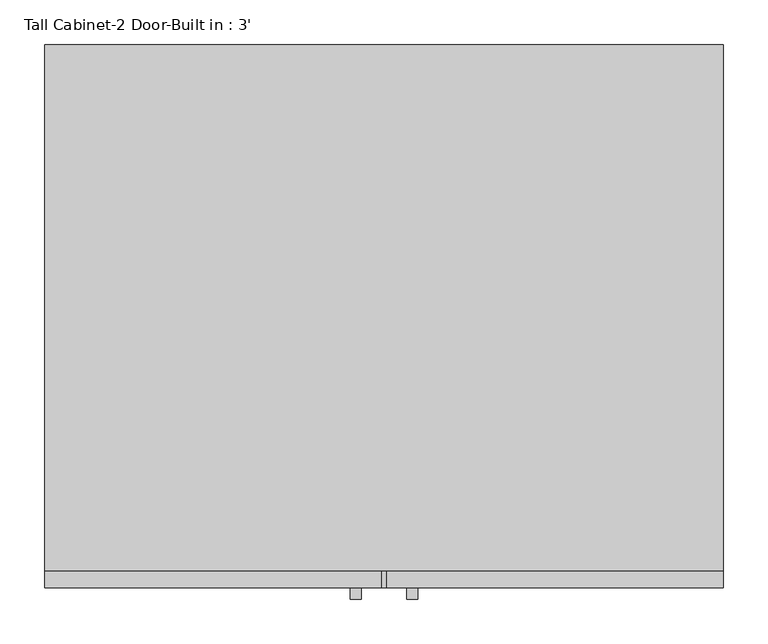
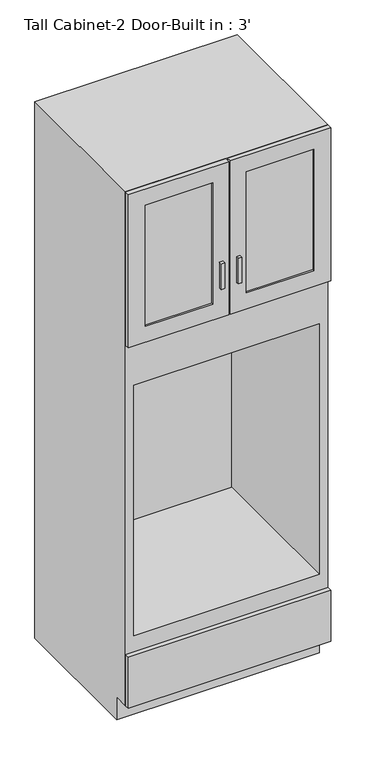
"""IFC4 building model written with IfcOpenShell, lengths in millimetres: furniture geometry, Tall Cabinet-2 Door-Built in : 3'."""

from ifc_helpers import new_model, si_unit, frame, origin, place, context, project, spatial, polyline, outline, extrude, faceted_brep, source, transform, mapped, element, save


def tall_cabinet_2_door_built_in_3_fb6977ac(model_context):
    return source(origin(), model_context, "Body", "SolidModel", [
        faceted_brep([(399.7377049, -590.55, 90.4875), (399.7377049, -590.55, 2135.1875), (-362.2622951, -590.55, 2135.1875), (-362.2622951, -590.55, 90.4875), (-343.2122951, -590.55, 2116.1375), (380.6877049, -590.55, 2116.1375), (380.6877049, -590.55, 1525.5875), (-343.2122951, -590.55, 1525.5875), (367.9877049, -590.55, 357.1875), (-330.5122951, -590.55, 357.1875), (-330.5122951, -590.55, 1354.1375), (367.9877049, -590.55, 1354.1375), (-362.2622951, 0.0, 2135.1875), (399.7377049, 0.0, 2135.1875), (399.7377049, 0.0, 0.0), (-362.2622951, 0.0, 0.0), (399.7377049, -533.4, 90.4875), (399.7377049, -533.4, 0.0), (-362.2622951, -533.4, 0.0), (-362.2622951, -533.4, 90.4875), (380.6877049, -19.05, 2116.1375), (380.6877049, -19.05, 1525.5875), (-343.2122951, -19.05, 1525.5875), (-343.2122951, -19.05, 2116.1375), (367.9877049, -19.05, 357.1875), (-330.5122951, -19.05, 357.1875), (-330.5122951, -19.05, 1354.1375), (367.9877049, -19.05, 1354.1375)], [[[0, 1, 2, 3], [4, 5, 6, 7], [8, 9, 10, 11]], [[12, 13, 14, 15]], [[1, 0, 16, 17, 14, 13]], [[2, 1, 13, 12]], [[3, 2, 12, 15, 18, 19]], [[0, 3, 19, 16]], [[6, 5, 20, 21]], [[4, 7, 22, 23]], [[5, 4, 23, 20]], [[14, 17, 18, 15]], [[18, 17, 16, 19]], [[7, 6, 21, 22]], [[9, 8, 24, 25]], [[10, 9, 25, 26]], [[11, 10, 26, 27]], [[8, 11, 27, 24]], [[21, 20, 23, 22]], [[25, 24, 27, 26]]]),
        extrude(outline(polyline([(399.7377049, -609.6), (-362.2622951, -609.6), (-362.2622951, -590.55), (399.7377049, -590.55), (399.7377049, -609.6)])), frame((0.0, 0.0, 90.4875), z_axis=(0.0, 0.0, 1.0), x_axis=(1.0, 0.0, 0.0)), (0.0, 0.0, 1.0), 203.2),
        extrude(outline(polyline([(2135.1875, 15.5627049), (2135.1875, -362.2622951), (1525.5875, -362.2622951), (1525.5875, 15.5627049), (2135.1875, 15.5627049)]), holes=[polyline([(2071.6875, -44.7622951), (1589.0875, -44.7622951), (1589.0875, -298.7622951), (2071.6875, -298.7622951), (2071.6875, -44.7622951)])]), frame((0.0, -609.6, 0.0), z_axis=(0.0, 1.0, 0.0), x_axis=(0.0, 0.0, 1.0)), (0.0, 0.0, 1.0), 19.05),
        extrude(outline(polyline([(2135.1875, 21.9127049), (1525.5875, 21.9127049), (1525.5875, 399.7377049), (2135.1875, 399.7377049), (2135.1875, 21.9127049)]), holes=[polyline([(2071.6875, 336.2377049), (1589.0875, 336.2377049), (1589.0875, 82.2377049), (2071.6875, 82.2377049), (2071.6875, 336.2377049)])]), frame((0.0, -609.6, 0.0), z_axis=(0.0, 1.0, 0.0), x_axis=(0.0, 0.0, 1.0)), (0.0, 0.0, 1.0), 19.05),
        extrude(outline(polyline([(399.7377049, -609.6), (-362.2622951, -609.6), (-362.2622951, -590.55), (399.7377049, -590.55), (399.7377049, -609.6)])), frame((0.0, 0.0, 90.4875), z_axis=(0.0, 0.0, 1.0), x_axis=(1.0, 0.0, 0.0)), (0.0, 0.0, 1.0), 203.2),
        extrude(outline(polyline([(-6.6622951, -622.3), (-19.1945267, -622.3), (-19.1945267, -609.6), (-6.6622951, -609.6), (-6.6622951, -622.3)])), frame((0.0, 0.0, 1645.6417867), z_axis=(0.0, 0.0, 1.0), x_axis=(1.0, 0.0, 0.0)), (0.0, 0.0, 1.0), 101.6),
        extrude(outline(polyline([(56.6699365, -622.3), (44.1377049, -622.3), (44.1377049, -609.6), (56.6699365, -609.6), (56.6699365, -622.3)])), frame((0.0, 0.0, 1645.6417867), z_axis=(0.0, 0.0, 1.0), x_axis=(1.0, 0.0, 0.0)), (0.0, 0.0, 1.0), 101.6),
        extrude(outline(polyline([(-44.7622951, -603.25), (-298.7622951, -603.25), (-298.7622951, -596.9), (-44.7622951, -596.9), (-44.7622951, -603.25)])), frame((0.0, 0.0, 1589.0875), z_axis=(0.0, 0.0, 1.0), x_axis=(1.0, 0.0, 0.0)), (0.0, 0.0, 1.0), 482.6),
        extrude(outline(polyline([(336.2377049, -603.25), (82.2377049, -603.25), (82.2377049, -596.9), (336.2377049, -596.9), (336.2377049, -603.25)])), frame((0.0, 0.0, 1589.0875), z_axis=(0.0, 0.0, 1.0), x_axis=(1.0, 0.0, 0.0)), (0.0, 0.0, 1.0), 482.6),
    ])


if __name__ == "__main__":
    model = new_model("IFC4")
    model_context = context("Model", 3, world=origin())
    ifc_project = project(units=[si_unit("LENGTHUNIT", "METRE", prefix="MILLI")], contexts=[model_context])
    site = spatial("IfcSite", under=ifc_project)
    building = spatial("IfcBuilding", under=site)
    placement = place(None, origin())
    tall_cabinet_2_door_built_in_3_shape = tall_cabinet_2_door_built_in_3_fb6977ac(model_context)
    element("IfcFurniture", 1, ObjectType="Tall Cabinet-2 Door-Built in : 3'", at=placement, inside=building, context=model_context, shape_type="MappedRepresentation", body=[
        mapped(tall_cabinet_2_door_built_in_3_shape, transform((0.0, 0.0, 0.0), x_axis=(1.0, 0.0, 0.0), y_axis=(0.0, 1.0, 0.0), z_axis=(0.0, 0.0, 1.0))),
    ])
    save(model, "model.ifc")

# Revit data of these elements
# Type "Tall Cabinet-2 Door-Built in : 3'"
#   Assembly Code = "C1030410"
#   Height = 7' - 0"
#   Depth = 2' - 0"
#   Height-Base of Built-in = 1' - 2"
#   Height-Built-in = 3' - 3 1/4"
#   Height-Upper Cabinet = 2' - 0"
#   Toe Depth = 0' - 3"
#   Toe Height = 0' - 3 1/2"
#   Width = 2' - 6"
#   Cabinet Material = none
#   Door/Drawer Material = none
#   Handle Material = Cabinets - Handles
#   Panel Material = Glass
#   Default Elevation = 0
#   Type Comments = ""
# Element 1 (IfcFurniture, "Tall Cabinet-2 Door-Built in : 3'")
#   Materials on its faces: "Cabinets", "Cabinets - Handles", "Glass"
# Materials
#   "Cabinets - Handles": class "Metal", colour RGB 57 57 57, transparency 0
#   "Glass": class "Glass", colour RGB 0 128 192, transparency 0.75, Description = "Soda Lime Glass", Cost = 0
#   "Cabinets": colour RGB 249 249 249, transparency 0
